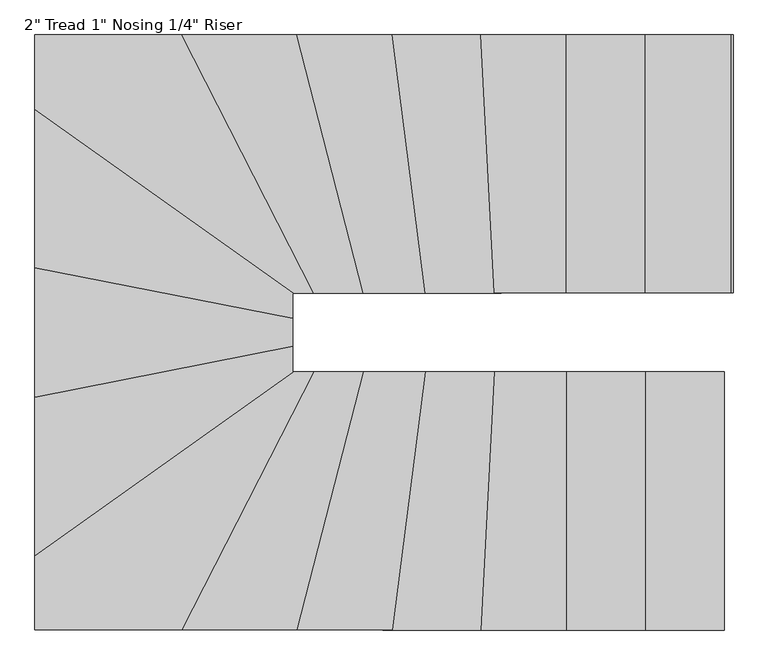
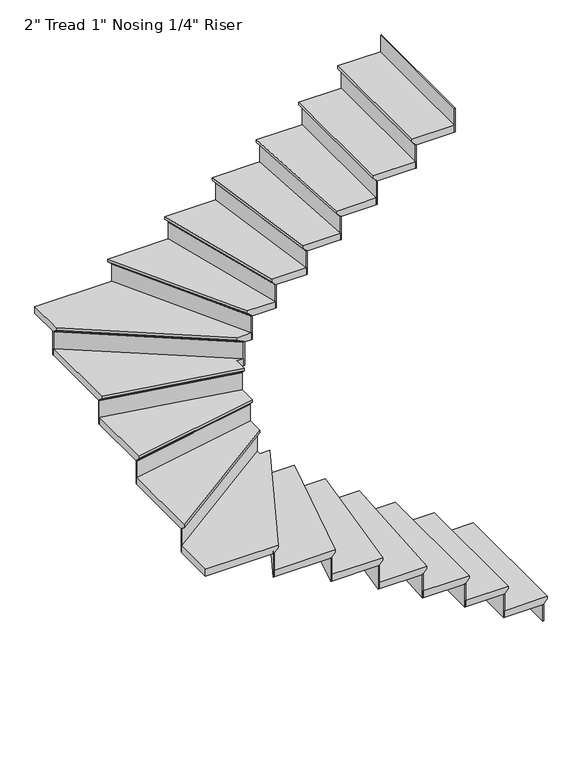
"""IFC4 building model written with IfcOpenShell, lengths in millimetres: stair flight geometry."""

from ifc_helpers import new_model, si_unit, origin, place, context, project, spatial, faceted_brep, source, transform, mapped, element, save


def stair_flight_c9f3f3be(model_context):
    return source(origin(), model_context, "Body", "Brep", [
        faceted_brep([(-7708.0614906, -9206.110779, 157.4131579), (-7708.0614906, -9206.110779, 176.4631579), (-7708.0614906, -10120.510779, 176.4631579), (-7708.0614906, -10120.510779, 157.4131579), (-7733.4614906, -9206.110779, 132.0131579), (-7733.4614906, -10120.510779, 132.0131579), (-8012.8614906, -9206.110779, 176.4631579), (-8012.8614906, -10120.510779, 176.4631579), (-7733.4614906, -10120.510779, 125.6631579), (-8012.8614906, -10120.510779, 125.6631579), (-8012.8614906, -9206.110779, 125.6631579), (-7733.4614906, -9206.110779, 125.6631579)], [[[0, 1, 2, 3]], [[4, 0, 3, 5]], [[2, 1, 6, 7]], [[8, 9, 10, 11]], [[2, 7, 9, 8, 5, 3]], [[8, 11, 4, 5]], [[6, 1, 0, 4, 11, 10]], [[7, 6, 10, 9]]]),
        faceted_brep([(-7733.4614906, -9206.110779, 125.6631579), (-7733.4614906, -9206.110779, 0.0), (-7739.8114906, -9206.110779, 0.0), (-7739.8114906, -9206.110779, 125.6631579), (-7733.4614906, -10120.510779, 125.6631579), (-7739.8114906, -10120.510779, 125.6631579), (-7739.8114906, -10120.510779, 0.0), (-7733.4614906, -10120.510779, 0.0)], [[[0, 1, 2, 3]], [[4, 5, 6, 7]], [[1, 0, 4, 7]], [[2, 1, 7, 6]], [[3, 2, 6, 5]], [[0, 3, 5, 4]]]),
        faceted_brep([(-8012.8614906, -9206.110779, 302.1263158), (-8012.8614906, -9206.110779, 125.6631579), (-8019.2114906, -9206.110779, 125.6631579), (-8019.2114906, -9206.110779, 302.1263158), (-8012.8614906, -10120.510779, 302.1263158), (-8019.2114906, -10120.510779, 302.1263158), (-8019.2114906, -10120.510779, 125.6631579), (-8012.8614906, -10120.510779, 125.6631579)], [[[0, 1, 2, 3]], [[4, 5, 6, 7]], [[1, 0, 4, 7]], [[2, 1, 7, 6]], [[3, 2, 6, 5]], [[0, 3, 5, 4]]]),
        faceted_brep([(-7987.4614906, -10120.510779, 352.9263158), (-7987.4614906, -9206.110779, 352.9263158), (-8292.2614906, -9206.110779, 352.9263158), (-8292.2614906, -10120.510779, 352.9263158), (-8012.8614906, -10120.510779, 302.1263158), (-8292.2614906, -10120.510779, 302.1263158), (-8292.2614906, -9206.110779, 302.1263158), (-8012.8614906, -9206.110779, 302.1263158), (-8012.8614906, -10120.510779, 308.4763158), (-7987.4614906, -10120.510779, 333.8763158), (-8012.8614906, -9206.110779, 308.4763158), (-7987.4614906, -9206.110779, 333.8763158)], [[[0, 1, 2, 3]], [[4, 5, 6, 7]], [[0, 3, 5, 4, 8, 9]], [[4, 7, 10, 8]], [[2, 1, 11, 10, 7, 6]], [[3, 2, 6, 5]], [[11, 1, 0, 9]], [[10, 11, 9, 8]]]),
        faceted_brep([(-8292.2614906, -9206.110779, 478.5894737), (-8292.2614906, -9206.110779, 302.1263158), (-8298.6114906, -9206.110779, 302.1263158), (-8298.6114906, -9206.110779, 478.5894737), (-8292.2614906, -10120.510779, 478.5894737), (-8298.6114906, -10120.510779, 478.5894737), (-8298.6114906, -10120.510779, 302.1263158), (-8292.2614906, -10120.510779, 302.1263158)], [[[0, 1, 2, 3]], [[4, 5, 6, 7]], [[1, 0, 4, 7]], [[2, 1, 7, 6]], [[3, 2, 6, 5]], [[0, 3, 5, 4]]]),
        faceted_brep([(-8266.8614906, -10120.510779, 529.3894737), (-8266.8614906, -9206.110779, 529.3894737), (-8547.928652, -9206.110779, 529.3894737), (-8595.4629224, -10120.510779, 529.3894737), (-8292.2614906, -10120.510779, 478.5894737), (-8595.4629224, -10120.510779, 478.5894737), (-8547.928652, -9206.110779, 478.5894737), (-8292.2614906, -9206.110779, 478.5894737), (-8292.2614906, -10120.510779, 484.9394737), (-8266.8614906, -10120.510779, 510.3394737), (-8292.2614906, -9206.110779, 484.9394737), (-8266.8614906, -9206.110779, 510.3394737)], [[[0, 1, 2, 3]], [[4, 5, 6, 7]], [[0, 3, 5, 4, 8, 9]], [[4, 7, 10, 8]], [[2, 1, 11, 10, 7, 6]], [[3, 2, 6, 5]], [[11, 1, 0, 9]], [[10, 11, 9, 8]]]),
        faceted_brep([(-8547.928652, -9206.110779, 655.0526316), (-8547.928652, -9206.110779, 478.5894737), (-8554.2872262, -9206.110779, 478.5894737), (-8554.2872262, -9206.110779, 655.0526316), (-8595.4629224, -10120.510779, 655.0526316), (-8601.8214966, -10120.510779, 655.0526316), (-8601.8214966, -10120.510779, 478.5894737), (-8595.4629224, -10120.510779, 478.5894737)], [[[0, 1, 2, 3]], [[4, 5, 6, 7]], [[1, 0, 4, 7]], [[2, 1, 7, 6]], [[3, 2, 6, 5]], [[0, 3, 5, 4]]]),
        faceted_brep([(-8570.0286258, -10120.510779, 705.8526316), (-8522.4943554, -9206.110779, 705.8526316), (-8792.0953519, -9206.110779, 705.8526316), (-8910.4514035, -10120.510779, 705.8526316), (-8595.4629224, -10120.510779, 655.0526316), (-8910.4514035, -10120.510779, 655.0526316), (-8792.0953519, -9206.110779, 655.0526316), (-8547.928652, -9206.110779, 655.0526316), (-8595.4629224, -10120.510779, 661.4026316), (-8570.0286258, -10120.510779, 686.8026316), (-8547.928652, -9206.110779, 661.4026316), (-8522.4943554, -9206.110779, 686.8026316)], [[[0, 1, 2, 3]], [[4, 5, 6, 7]], [[0, 3, 5, 4, 8, 9]], [[4, 7, 10, 8]], [[2, 1, 11, 10, 7, 6]], [[3, 2, 6, 5]], [[11, 1, 0, 9]], [[10, 11, 9, 8]]]),
        faceted_brep([(-8792.0953519, -9206.110779, 831.5157895), (-8792.0953519, -9206.110779, 655.0526316), (-8798.4983236, -9206.110779, 655.0526316), (-8798.4983236, -9206.110779, 831.5157895), (-8910.4514035, -10120.510779, 831.5157895), (-8916.8543753, -10120.510779, 831.5157895), (-8916.8543753, -10120.510779, 655.0526316), (-8910.4514035, -10120.510779, 655.0526316)], [[[0, 1, 2, 3]], [[4, 5, 6, 7]], [[1, 0, 4, 7]], [[2, 1, 7, 6]], [[3, 2, 6, 5]], [[0, 3, 5, 4]]]),
        faceted_brep([(-8884.8395164, -10120.510779, 882.3157895), (-8766.4834647, -9206.110779, 882.3157895), (-9013.7225743, -9206.110779, 882.3157895), (-9248.8530217, -10120.510779, 882.3157895), (-8910.4514035, -10120.510779, 831.5157895), (-9248.8530217, -10120.510779, 831.5157895), (-9013.7225743, -9206.110779, 831.5157895), (-8792.0953519, -9206.110779, 831.5157895), (-8910.4514035, -10120.510779, 837.8657895), (-8884.8395164, -10120.510779, 863.2657895), (-8792.0953519, -9206.110779, 837.8657895), (-8766.4834647, -9206.110779, 863.2657895)], [[[0, 1, 2, 3]], [[4, 5, 6, 7]], [[0, 3, 5, 4, 8, 9]], [[4, 7, 10, 8]], [[2, 1, 11, 10, 7, 6]], [[3, 2, 6, 5]], [[11, 1, 0, 9]], [[10, 11, 9, 8]]]),
        faceted_brep([(-9013.7225743, -9206.110779, 1007.9789474), (-9013.7225743, -9206.110779, 831.5157895), (-9020.2791512, -9206.110779, 831.5157895), (-9020.2791512, -9206.110779, 1007.9789474), (-9248.8530217, -10120.510779, 1007.9789474), (-9255.4095986, -10120.510779, 1007.9789474), (-9255.4095986, -10120.510779, 831.5157895), (-9248.8530217, -10120.510779, 831.5157895)], [[[0, 1, 2, 3]], [[4, 5, 6, 7]], [[1, 0, 4, 7]], [[2, 1, 7, 6]], [[3, 2, 6, 5]], [[0, 3, 5, 4]]]),
        faceted_brep([(-9222.6267143, -10120.510779, 1058.7789474), (-8987.4962669, -9206.110779, 1058.7789474), (-9190.0692104, -9206.110779, 1058.7789474), (-9658.8938317, -10120.510779, 1058.7789474), (-9248.8530217, -10120.510779, 1007.9789474), (-9658.8938317, -10120.510779, 1007.9789474), (-9190.0692104, -9206.110779, 1007.9789474), (-9013.7225743, -9206.110779, 1007.9789474), (-9248.8530217, -10120.510779, 1014.3289474), (-9222.6267143, -10120.510779, 1039.7289474), (-9013.7225743, -9206.110779, 1014.3289474), (-8987.4962669, -9206.110779, 1039.7289474)], [[[0, 1, 2, 3]], [[4, 5, 6, 7]], [[0, 3, 5, 4, 8, 9]], [[4, 7, 10, 8]], [[2, 1, 11, 10, 7, 6]], [[3, 2, 6, 5]], [[11, 1, 0, 9]], [[10, 11, 9, 8]]]),
        faceted_brep([(-9190.0692104, -9206.110779, 1184.4421053), (-9190.0692104, -9206.110779, 1007.9789474), (-9197.2051936, -9206.110779, 1007.9789474), (-9197.2051936, -9206.110779, 1184.4421053), (-9658.8938317, -10120.510779, 1184.4421053), (-9666.0298149, -10120.510779, 1184.4421053), (-9666.0298149, -10120.510779, 1007.9789474), (-9658.8938317, -10120.510779, 1007.9789474)], [[[0, 1, 2, 3]], [[4, 5, 6, 7]], [[1, 0, 4, 7]], [[2, 1, 7, 6]], [[3, 2, 6, 5]], [[0, 3, 5, 4]]]),
        faceted_brep([(-10150.1931824, -9826.8296453, 1235.2421053), (-10150.1931824, -10120.510779, 1235.2421053), (-9630.3498992, -10120.510779, 1235.2421053), (-9161.5252779, -9206.110779, 1235.2421053), (-9235.7931824, -9206.110779, 1235.2421053), (-9235.7931824, -9176.5556961, 1235.2421053), (-10150.1931824, -10120.510779, 1184.4421053), (-10150.1931824, -9826.8296453, 1184.4421053), (-9235.7931824, -9176.5556961, 1184.4421053), (-9235.7931824, -9206.110779, 1184.4421053), (-9190.0692104, -9206.110779, 1184.4421053), (-9658.8938317, -10120.510779, 1184.4421053), (-9658.8938317, -10120.510779, 1190.7921053), (-9630.3498992, -10120.510779, 1216.1921053), (-9190.0692104, -9206.110779, 1190.7921053), (-9161.5252779, -9206.110779, 1216.1921053)], [[[0, 1, 2, 3, 4, 5]], [[6, 7, 8, 9, 10, 11]], [[1, 0, 7, 6]], [[2, 1, 6, 11, 12, 13]], [[11, 10, 14, 12]], [[4, 3, 15, 14, 10, 9]], [[5, 4, 9, 8]], [[0, 5, 8, 7]], [[15, 3, 2, 13]], [[14, 15, 13, 12]]]),
        faceted_brep([(-9235.7931824, -9176.5556961, 1360.9052632), (-9235.7931824, -9176.5556961, 1184.4421053), (-9235.7931824, -9168.7637213, 1184.4421053), (-9235.7931824, -9168.7637213, 1360.9052632), (-10150.1931824, -9826.8296453, 1360.9052632), (-10150.1931824, -9819.0376705, 1360.9052632), (-10150.1931824, -9819.0376705, 1184.4421053), (-10150.1931824, -9826.8296453, 1184.4421053)], [[[0, 1, 2, 3]], [[4, 5, 6, 7]], [[1, 0, 4, 7]], [[2, 1, 7, 6]], [[3, 2, 6, 5]], [[0, 3, 5, 4]]]),
        faceted_brep([(-10150.1931824, -9857.9975445, 1411.7052632), (-9235.7931824, -9207.7235953, 1411.7052632), (-9235.7931824, -9090.1016091, 1411.7052632), (-10150.1931824, -9270.3424654, 1411.7052632), (-10150.1931824, -9826.8296453, 1360.9052632), (-10150.1931824, -9270.3424654, 1360.9052632), (-9235.7931824, -9090.1016091, 1360.9052632), (-9235.7931824, -9176.5556961, 1360.9052632), (-10150.1931824, -9826.8296453, 1367.2552632), (-10150.1931824, -9857.9975445, 1392.6552632), (-9235.7931824, -9176.5556961, 1367.2552632), (-9235.7931824, -9207.7235953, 1392.6552632)], [[[0, 1, 2, 3]], [[4, 5, 6, 7]], [[0, 3, 5, 4, 8, 9]], [[4, 7, 10, 8]], [[2, 1, 11, 10, 7, 6]], [[3, 2, 6, 5]], [[11, 1, 0, 9]], [[10, 11, 9, 8]]]),
        faceted_brep([(-9235.7931824, -9090.1016091, 1537.3684211), (-9235.7931824, -9090.1016091, 1360.9052632), (-9235.7931824, -9083.6294236, 1360.9052632), (-9235.7931824, -9083.6294236, 1537.3684211), (-10150.1931824, -9270.3424654, 1537.3684211), (-10150.1931824, -9263.87028, 1537.3684211), (-10150.1931824, -9263.87028, 1360.9052632), (-10150.1931824, -9270.3424654, 1360.9052632)], [[[0, 1, 2, 3]], [[4, 5, 6, 7]], [[1, 0, 4, 7]], [[2, 1, 7, 6]], [[3, 2, 6, 5]], [[0, 3, 5, 4]]]),
        faceted_brep([(-10150.1931824, -9296.2312071, 1588.1684211), (-9235.7931824, -9115.9903508, 1588.1684211), (-9235.7931824, -8990.9424654, 1588.1684211), (-10150.1931824, -8810.7016091, 1588.1684211), (-10150.1931824, -9270.3424654, 1537.3684211), (-10150.1931824, -8810.7016091, 1537.3684211), (-9235.7931824, -8990.9424654, 1537.3684211), (-9235.7931824, -9090.1016091, 1537.3684211), (-10150.1931824, -9270.3424654, 1543.7184211), (-10150.1931824, -9296.2312071, 1569.1184211), (-9235.7931824, -9090.1016091, 1543.7184211), (-9235.7931824, -9115.9903508, 1569.1184211)], [[[0, 1, 2, 3]], [[4, 5, 6, 7]], [[0, 3, 5, 4, 8, 9]], [[4, 7, 10, 8]], [[2, 1, 11, 10, 7, 6]], [[3, 2, 6, 5]], [[11, 1, 0, 9]], [[10, 11, 9, 8]]]),
        faceted_brep([(-9235.7931824, -8990.9424654, 1713.8315789), (-9235.7931824, -8990.9424654, 1537.3684211), (-9235.7931824, -8984.47028, 1537.3684211), (-9235.7931824, -8984.47028, 1713.8315789), (-10150.1931824, -8810.7016091, 1713.8315789), (-10150.1931824, -8804.2294236, 1713.8315789), (-10150.1931824, -8804.2294236, 1537.3684211), (-10150.1931824, -8810.7016091, 1537.3684211)], [[[0, 1, 2, 3]], [[4, 5, 6, 7]], [[1, 0, 4, 7]], [[2, 1, 7, 6]], [[3, 2, 6, 5]], [[0, 3, 5, 4]]]),
        faceted_brep([(-10150.1931824, -8836.5903508, 1764.6315789), (-9235.7931824, -9016.8312071, 1764.6315789), (-9235.7931824, -8926.710779, 1764.6315789), (-9189.6977079, -8926.710779, 1764.6315789), (-10150.1931824, -8243.6561143, 1764.6315789), (-10150.1931824, -8810.7016091, 1713.8315789), (-10150.1931824, -8243.6561143, 1713.8315789), (-9189.6977079, -8926.710779, 1713.8315789), (-9235.7931824, -8926.710779, 1713.8315789), (-9235.7931824, -8990.9424654, 1713.8315789), (-10150.1931824, -8810.7016091, 1720.1815789), (-10150.1931824, -8836.5903508, 1745.5815789), (-9235.7931824, -8990.9424654, 1720.1815789), (-9235.7931824, -9016.8312071, 1745.5815789)], [[[0, 1, 2, 3, 4]], [[5, 6, 7, 8, 9]], [[0, 4, 6, 5, 10, 11]], [[5, 9, 12, 10]], [[2, 1, 13, 12, 9, 8]], [[3, 2, 8, 7]], [[4, 3, 7, 6]], [[13, 1, 0, 11]], [[12, 13, 11, 10]]]),
        faceted_brep([(-9189.6977079, -8926.710779, 1890.2947368), (-9189.6977079, -8926.710779, 1713.8315789), (-9178.7408154, -8926.710779, 1713.8315789), (-9178.7408154, -8926.710779, 1890.2947368), (-10150.1931824, -8243.6561143, 1890.2947368), (-10150.1931824, -8235.8641395, 1890.2947368), (-10150.1931824, -8235.8641395, 1713.8315789), (-10150.1931824, -8243.6561143, 1713.8315789)], [[[0, 1, 2, 3]], [[4, 5, 6, 7]], [[1, 0, 4, 7]], [[2, 1, 7, 6]], [[3, 2, 6, 5]], [[0, 3, 5, 4]]]),
        faceted_brep([(-9601.8059667, -8012.310779, 1941.0947368), (-10150.1931824, -8012.310779, 1941.0947368), (-10150.1931824, -8274.8240135, 1941.0947368), (-9233.5252779, -8926.710779, 1941.0947368), (-9132.9813454, -8926.710779, 1941.0947368), (-10150.1931824, -8012.310779, 1890.2947368), (-9601.8059667, -8012.310779, 1890.2947368), (-9132.9813454, -8926.710779, 1890.2947368), (-9189.6977079, -8926.710779, 1890.2947368), (-10150.1931824, -8243.6561143, 1890.2947368), (-10150.1931824, -8243.6561143, 1896.6447368), (-10150.1931824, -8274.8240135, 1922.0447368), (-9189.6977079, -8926.710779, 1896.6447368), (-9233.5252779, -8926.710779, 1922.0447368)], [[[0, 1, 2, 3, 4]], [[5, 6, 7, 8, 9]], [[1, 0, 6, 5]], [[2, 1, 5, 9, 10, 11]], [[9, 8, 12, 10]], [[4, 3, 13, 12, 8, 7]], [[0, 4, 7, 6]], [[13, 3, 2, 11]], [[12, 13, 11, 10]]]),
        faceted_brep([(-9132.9813454, -8926.710779, 2066.7578947), (-9132.9813454, -8926.710779, 1890.2947368), (-9125.8453622, -8926.710779, 1890.2947368), (-9125.8453622, -8926.710779, 2066.7578947), (-9601.8059667, -8012.310779, 2066.7578947), (-9594.6699835, -8012.310779, 2066.7578947), (-9594.6699835, -8012.310779, 1890.2947368), (-9601.8059667, -8012.310779, 1890.2947368)], [[[0, 1, 2, 3]], [[4, 5, 6, 7]], [[1, 0, 4, 7]], [[2, 1, 7, 6]], [[3, 2, 6, 5]], [[0, 3, 5, 4]]]),
        faceted_brep([(-9630.3498992, -8012.310779, 2117.5578947), (-9161.5252779, -8926.710779, 2117.5578947), (-8961.2699594, -8926.710779, 2117.5578947), (-9196.4004068, -8012.310779, 2117.5578947), (-9601.8059667, -8012.310779, 2066.7578947), (-9196.4004068, -8012.310779, 2066.7578947), (-8961.2699594, -8926.710779, 2066.7578947), (-9132.9813454, -8926.710779, 2066.7578947), (-9601.8059667, -8012.310779, 2073.1078947), (-9630.3498992, -8012.310779, 2098.5078947), (-9132.9813454, -8926.710779, 2073.1078947), (-9161.5252779, -8926.710779, 2098.5078947)], [[[0, 1, 2, 3]], [[4, 5, 6, 7]], [[0, 3, 5, 4, 8, 9]], [[4, 7, 10, 8]], [[2, 1, 11, 10, 7, 6]], [[3, 2, 6, 5]], [[11, 1, 0, 9]], [[10, 11, 9, 8]]]),
        faceted_brep([(-8961.2699594, -8926.710779, 2243.2210526), (-8961.2699594, -8926.710779, 2066.7578947), (-8954.7133825, -8926.710779, 2066.7578947), (-8954.7133825, -8926.710779, 2243.2210526), (-9196.4004068, -8012.310779, 2243.2210526), (-9189.84383, -8012.310779, 2243.2210526), (-9189.84383, -8012.310779, 2066.7578947), (-9196.4004068, -8012.310779, 2066.7578947)], [[[0, 1, 2, 3]], [[4, 5, 6, 7]], [[1, 0, 4, 7]], [[2, 1, 7, 6]], [[3, 2, 6, 5]], [[0, 3, 5, 4]]]),
        faceted_brep([(-9222.6267143, -8012.310779, 2294.0210526), (-8987.4962669, -8926.710779, 2294.0210526), (-8740.8715776, -8926.710779, 2294.0210526), (-8859.2276293, -8012.310779, 2294.0210526), (-9196.4004068, -8012.310779, 2243.2210526), (-8859.2276293, -8012.310779, 2243.2210526), (-8740.8715776, -8926.710779, 2243.2210526), (-8961.2699594, -8926.710779, 2243.2210526), (-9196.4004068, -8012.310779, 2249.5710526), (-9222.6267143, -8012.310779, 2274.9710526), (-8961.2699594, -8926.710779, 2249.5710526), (-8987.4962669, -8926.710779, 2274.9710526)], [[[0, 1, 2, 3]], [[4, 5, 6, 7]], [[0, 3, 5, 4, 8, 9]], [[4, 7, 10, 8]], [[2, 1, 11, 10, 7, 6]], [[3, 2, 6, 5]], [[11, 1, 0, 9]], [[10, 11, 9, 8]]]),
        faceted_brep([(-8740.8715776, -8926.710779, 2419.6842105), (-8740.8715776, -8926.710779, 2243.2210526), (-8734.4686059, -8926.710779, 2243.2210526), (-8734.4686059, -8926.710779, 2419.6842105), (-8859.2276293, -8012.310779, 2419.6842105), (-8852.8246575, -8012.310779, 2419.6842105), (-8852.8246575, -8012.310779, 2243.2210526), (-8859.2276293, -8012.310779, 2243.2210526)], [[[0, 1, 2, 3]], [[4, 5, 6, 7]], [[1, 0, 4, 7]], [[2, 1, 7, 6]], [[3, 2, 6, 5]], [[0, 3, 5, 4]]]),
        faceted_brep([(-8884.8395164, -8012.310779, 2470.4842105), (-8766.4834647, -8926.710779, 2470.4842105), (-8497.0600587, -8926.710779, 2470.4842105), (-8544.5943291, -8012.310779, 2470.4842105), (-8859.2276293, -8012.310779, 2419.6842105), (-8544.5943291, -8012.310779, 2419.6842105), (-8497.0600587, -8926.710779, 2419.6842105), (-8740.8715776, -8926.710779, 2419.6842105), (-8859.2276293, -8012.310779, 2426.0342105), (-8884.8395164, -8012.310779, 2451.4342105), (-8740.8715776, -8926.710779, 2426.0342105), (-8766.4834647, -8926.710779, 2451.4342105)], [[[0, 1, 2, 3]], [[4, 5, 6, 7]], [[0, 3, 5, 4, 8, 9]], [[4, 7, 10, 8]], [[2, 1, 11, 10, 7, 6]], [[3, 2, 6, 5]], [[11, 1, 0, 9]], [[10, 11, 9, 8]]]),
        faceted_brep([(-8497.0600587, -8926.710779, 2596.1473684), (-8497.0600587, -8926.710779, 2419.6842105), (-8490.7014845, -8926.710779, 2419.6842105), (-8490.7014845, -8926.710779, 2596.1473684), (-8544.5943291, -8012.310779, 2596.1473684), (-8538.235755, -8012.310779, 2596.1473684), (-8538.235755, -8012.310779, 2419.6842105), (-8544.5943291, -8012.310779, 2419.6842105)], [[[0, 1, 2, 3]], [[4, 5, 6, 7]], [[1, 0, 4, 7]], [[2, 1, 7, 6]], [[3, 2, 6, 5]], [[0, 3, 5, 4]]]),
        faceted_brep([(-8570.0286258, -8012.310779, 2646.9473684), (-8522.4943554, -8926.710779, 2646.9473684), (-8241.4614906, -8926.710779, 2646.9473684), (-8241.4614906, -8012.310779, 2646.9473684), (-8544.5943291, -8012.310779, 2596.1473684), (-8241.4614906, -8012.310779, 2596.1473684), (-8241.4614906, -8926.710779, 2596.1473684), (-8497.0600587, -8926.710779, 2596.1473684), (-8544.5943291, -8012.310779, 2602.4973684), (-8570.0286258, -8012.310779, 2627.8973684), (-8497.0600587, -8926.710779, 2602.4973684), (-8522.4943554, -8926.710779, 2627.8973684)], [[[0, 1, 2, 3]], [[4, 5, 6, 7]], [[0, 3, 5, 4, 8, 9]], [[4, 7, 10, 8]], [[2, 1, 11, 10, 7, 6]], [[3, 2, 6, 5]], [[11, 1, 0, 9]], [[10, 11, 9, 8]]]),
        faceted_brep([(-8241.4614906, -8926.710779, 2772.6105263), (-8241.4614906, -8926.710779, 2596.1473684), (-8235.1114906, -8926.710779, 2596.1473684), (-8235.1114906, -8926.710779, 2772.6105263), (-8241.4614906, -8012.310779, 2772.6105263), (-8235.1114906, -8012.310779, 2772.6105263), (-8235.1114906, -8012.310779, 2596.1473684), (-8241.4614906, -8012.310779, 2596.1473684)], [[[0, 1, 2, 3]], [[4, 5, 6, 7]], [[1, 0, 4, 7]], [[2, 1, 7, 6]], [[3, 2, 6, 5]], [[0, 3, 5, 4]]]),
        faceted_brep([(-8266.8614906, -8012.310779, 2823.4105263), (-8266.8614906, -8926.710779, 2823.4105263), (-7962.0614906, -8926.710779, 2823.4105263), (-7962.0614906, -8012.310779, 2823.4105263), (-8241.4614906, -8012.310779, 2772.6105263), (-7962.0614906, -8012.310779, 2772.6105263), (-7962.0614906, -8926.710779, 2772.6105263), (-8241.4614906, -8926.710779, 2772.6105263), (-8241.4614906, -8012.310779, 2778.9605263), (-8266.8614906, -8012.310779, 2804.3605263), (-8241.4614906, -8926.710779, 2778.9605263), (-8266.8614906, -8926.710779, 2804.3605263)], [[[0, 1, 2, 3]], [[4, 5, 6, 7]], [[0, 3, 5, 4, 8, 9]], [[4, 7, 10, 8]], [[2, 1, 11, 10, 7, 6]], [[3, 2, 6, 5]], [[11, 1, 0, 9]], [[10, 11, 9, 8]]]),
        faceted_brep([(-7962.0614906, -8926.710779, 2949.0736842), (-7962.0614906, -8926.710779, 2772.6105263), (-7955.7114906, -8926.710779, 2772.6105263), (-7955.7114906, -8926.710779, 2949.0736842), (-7962.0614906, -8012.310779, 2949.0736842), (-7955.7114906, -8012.310779, 2949.0736842), (-7955.7114906, -8012.310779, 2772.6105263), (-7962.0614906, -8012.310779, 2772.6105263)], [[[0, 1, 2, 3]], [[4, 5, 6, 7]], [[1, 0, 4, 7]], [[2, 1, 7, 6]], [[3, 2, 6, 5]], [[0, 3, 5, 4]]]),
        faceted_brep([(-7682.6614906, -8926.710779, 3125.5368421), (-7682.6614906, -8926.710779, 2949.0736842), (-7676.3114906, -8926.710779, 2949.0736842), (-7676.3114906, -8926.710779, 3125.5368421), (-7682.6614906, -8012.310779, 3125.5368421), (-7676.3114906, -8012.310779, 3125.5368421), (-7676.3114906, -8012.310779, 2949.0736842), (-7682.6614906, -8012.310779, 2949.0736842)], [[[0, 1, 2, 3]], [[4, 5, 6, 7]], [[1, 0, 4, 7]], [[2, 1, 7, 6]], [[3, 2, 6, 5]], [[0, 3, 5, 4]]]),
        faceted_brep([(-7987.4614906, -8012.310779, 2999.8736842), (-7987.4614906, -8926.710779, 2999.8736842), (-7682.6614906, -8926.710779, 2999.8736842), (-7682.6614906, -8012.310779, 2999.8736842), (-7962.0614906, -8012.310779, 2949.0736842), (-7682.6614906, -8012.310779, 2949.0736842), (-7682.6614906, -8926.710779, 2949.0736842), (-7962.0614906, -8926.710779, 2949.0736842), (-7962.0614906, -8012.310779, 2955.4236842), (-7987.4614906, -8012.310779, 2980.8236842), (-7962.0614906, -8926.710779, 2955.4236842), (-7987.4614906, -8926.710779, 2980.8236842)], [[[0, 1, 2, 3]], [[4, 5, 6, 7]], [[0, 3, 5, 4, 8, 9]], [[4, 7, 10, 8]], [[2, 1, 11, 10, 7, 6]], [[3, 2, 6, 5]], [[11, 1, 0, 9]], [[10, 11, 9, 8]]]),
    ])


if __name__ == "__main__":
    model = new_model("IFC4")
    model_context = context("Model", 3, world=origin())
    ifc_project = project(units=[si_unit("LENGTHUNIT", "METRE", prefix="MILLI")], contexts=[model_context])
    site = spatial("IfcSite", under=ifc_project)
    building = spatial("IfcBuilding", under=site)
    placement = place(None, origin())
    stair_flight_shape = stair_flight_c9f3f3be(model_context)
    element("IfcStairFlight", 1, ObjectType="2\" Tread 1\" Nosing 1/4\" Riser", at=placement, inside=building, context=model_context, shape_type="MappedRepresentation", body=[
        mapped(stair_flight_shape, transform((0.0, 0.0, 0.0), x_axis=(1.0, 0.0, 0.0), y_axis=(0.0, 1.0, 0.0), z_axis=(0.0, 0.0, 1.0))),
    ])
    save(model, "model.ifc")
